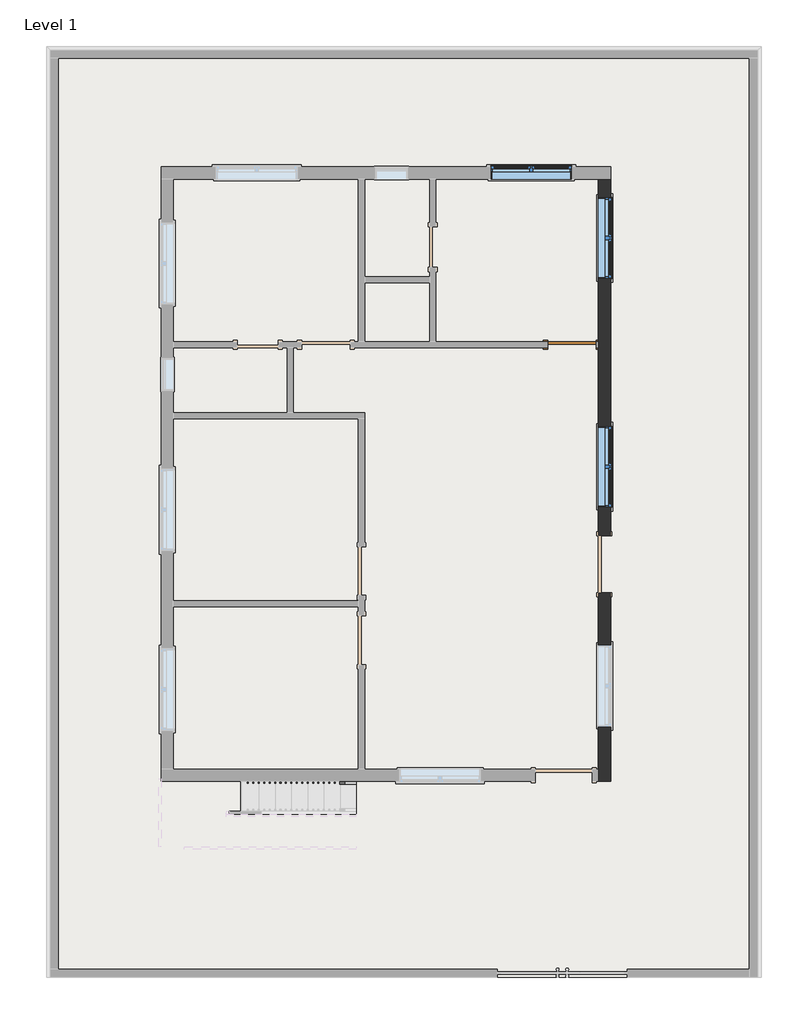
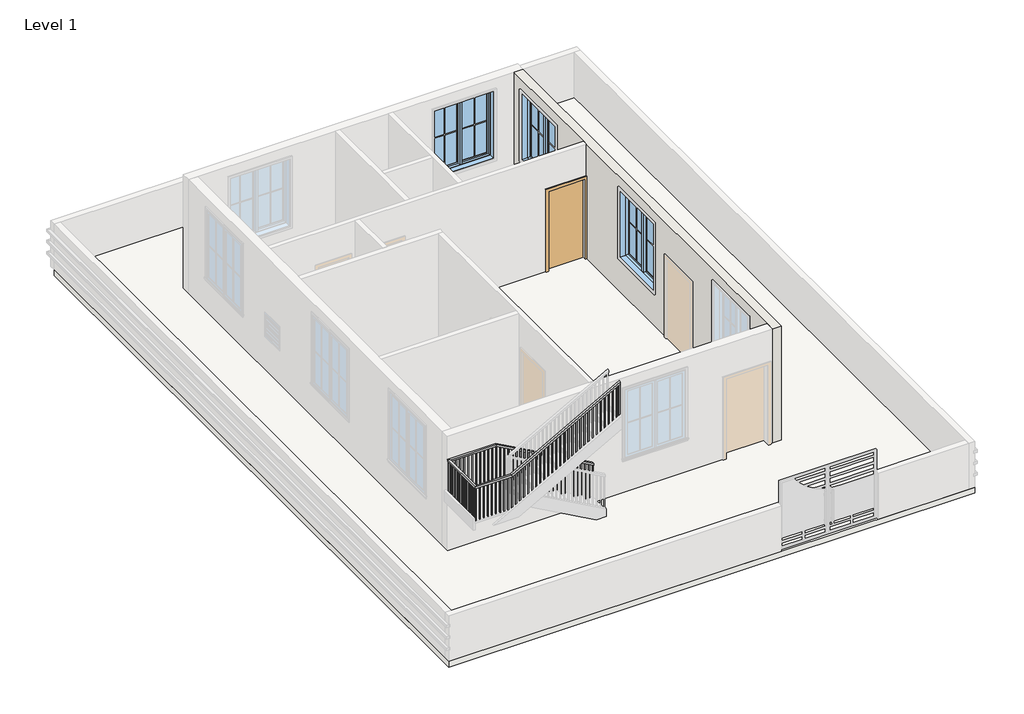
# One storey, part 2 of 3: 3 windows, 1 door, 1 railing, 1 slab, 1 wall.
"""IFC4 building model written with IfcOpenShell, lengths in millimetres."""

from ifc_helpers import new_model, si_unit, frame, origin, place, context, project, spatial, polyline, outline, extrude, faceted_brep, transform, mapped, element, save
from components import single_flush_door_3_e5f9f3c4, window_casement_double_win_5_f93960c7

model = new_model("IFC4")

# Units and contexts
model_context = context("Model", 3, world=origin())
ifc_project = project(units=[si_unit("LENGTHUNIT", "METRE", prefix="MILLI")], contexts=[model_context])

# Site, building, storey
site = spatial("IfcSite", under=ifc_project)
building = spatial("IfcBuilding", under=site)
storey = spatial("IfcBuildingStorey", under=building, Name="Level 1", Elevation=0.0)

# Door
placement = place(None, origin())
single_flush_door_3_shape = single_flush_door_3_e5f9f3c4(model_context)
element("IfcDoor", 1, ObjectType="Single-Flush : DOOR 3'", at=placement, inside=storey, context=model_context, shape_type="MappedRepresentation", body=[
    mapped(single_flush_door_3_shape, transform((2232.6801431, 2878.7566963, 0.0), x_axis=(1.0, 0.0, 0.0), y_axis=(0.0, 1.0, 0.0), z_axis=(0.0, 0.0, 1.0))),
])

# Railing
element("IfcRailing", 2, ObjectType="Handrail - Rectangular", at=placement, inside=storey, context=model_context, shape_type="SolidModel", body=[
    faceted_brep([(-1805.9198569, -5357.1933037, 1083.7333333), (-1805.9198569, -5357.1933037, 1025.620221), (-1805.9198569, -5306.3933037, 1025.620221), (-1805.9198569, -5306.3933037, 1083.7333333), (-4244.3198569, -5357.1933037, 2438.4), (-4257.4834592, -5357.1933037, 2387.6), (-4257.4834592, -5306.3933037, 2387.6), (-4244.3198569, -5306.3933037, 2438.4), (-5412.7198569, -5357.1933037, 2438.4), (-5412.7198569, -5357.1933037, 2387.6), (-5463.5198569, -5306.3933037, 2387.6), (-5463.5198569, -5306.3933037, 2438.4), (-5412.7198569, -6474.7933037, 2438.4), (-5412.7198569, -6474.7933037, 2387.6), (-5463.5198569, -6525.5933037, 2387.6), (-5463.5198569, -6525.5933037, 2438.4), (-4549.1198569, -6474.7933037, 2438.4), (-4535.9562547, -6474.7933037, 2387.6), (-4535.9562547, -6525.5933037, 2387.6), (-4549.1198569, -6525.5933037, 2438.4), (-1805.9198569, -6474.7933037, 3962.4), (-1805.9198569, -6525.5933037, 3962.4), (-1805.9198569, -6525.5933037, 3904.2868876), (-1805.9198569, -6474.7933037, 3904.2868876)], [[[0, 1, 2, 3]], [[1, 0, 4, 5]], [[2, 1, 5, 6]], [[3, 2, 6, 7]], [[0, 3, 7, 4]], [[5, 4, 8, 9]], [[6, 5, 9, 10]], [[7, 6, 10, 11]], [[4, 7, 11, 8]], [[9, 8, 12, 13]], [[10, 9, 13, 14]], [[11, 10, 14, 15]], [[8, 11, 15, 12]], [[13, 12, 16, 17]], [[14, 13, 17, 18]], [[15, 14, 18, 19]], [[12, 15, 19, 16]], [[20, 21, 22, 23]], [[17, 16, 20, 23]], [[18, 17, 23, 22]], [[19, 18, 22, 21]], [[16, 19, 21, 20]]]),
    extrude(outline(polyline([(3867.245221, -1872.5948569), (3856.6618876, -1891.6448569), (2878.6666667, -1891.6448569), (2878.6666667, -1872.5948569), (3867.245221, -1872.5948569)])), frame((0.0, -6509.7183037, 0.0), z_axis=(0.0, 1.0, 0.0), x_axis=(0.0, 0.0, 1.0)), (0.0, 0.0, 1.0), 19.05),
    extrude(outline(polyline([(3810.8007765, -1974.1948569), (3800.2174432, -1993.2448569), (2878.6666667, -1993.2448569), (2878.6666667, -1974.1948569), (3810.8007765, -1974.1948569)])), frame((0.0, -6509.7183037, 0.0), z_axis=(0.0, 1.0, 0.0), x_axis=(0.0, 0.0, 1.0)), (0.0, 0.0, 1.0), 19.05),
    extrude(outline(polyline([(3754.3563321, -2075.7948569), (3743.7729988, -2094.8448569), (2878.6666667, -2094.8448569), (2878.6666667, -2075.7948569), (3754.3563321, -2075.7948569)])), frame((0.0, -6509.7183037, 0.0), z_axis=(0.0, 1.0, 0.0), x_axis=(0.0, 0.0, 1.0)), (0.0, 0.0, 1.0), 19.05),
    extrude(outline(polyline([(3697.9118876, -2177.3948569), (3687.3285543, -2196.4448569), (2709.3333333, -2196.4448569), (2709.3333333, -2177.3948569), (3697.9118876, -2177.3948569)])), frame((0.0, -6509.7183037, 0.0), z_axis=(0.0, 1.0, 0.0), x_axis=(0.0, 0.0, 1.0)), (0.0, 0.0, 1.0), 19.05),
    extrude(outline(polyline([(3641.4674432, -2278.9948569), (3630.8841099, -2298.0448569), (2709.3333333, -2298.0448569), (2709.3333333, -2278.9948569), (3641.4674432, -2278.9948569)])), frame((0.0, -6509.7183037, 0.0), z_axis=(0.0, 1.0, 0.0), x_axis=(0.0, 0.0, 1.0)), (0.0, 0.0, 1.0), 19.05),
    extrude(outline(polyline([(3585.0229988, -2380.5948569), (3574.4396654, -2399.6448569), (2709.3333333, -2399.6448569), (2709.3333333, -2380.5948569), (3585.0229988, -2380.5948569)])), frame((0.0, -6509.7183037, 0.0), z_axis=(0.0, 1.0, 0.0), x_axis=(0.0, 0.0, 1.0)), (0.0, 0.0, 1.0), 19.05),
    extrude(outline(polyline([(3528.5785543, -2482.1948569), (3517.995221, -2501.2448569), (2540.0, -2501.2448569), (2540.0, -2482.1948569), (3528.5785543, -2482.1948569)])), frame((0.0, -6509.7183037, 0.0), z_axis=(0.0, 1.0, 0.0), x_axis=(0.0, 0.0, 1.0)), (0.0, 0.0, 1.0), 19.05),
    extrude(outline(polyline([(3472.1341099, -2583.7948569), (3461.5507765, -2602.8448569), (2540.0, -2602.8448569), (2540.0, -2583.7948569), (3472.1341099, -2583.7948569)])), frame((0.0, -6509.7183037, 0.0), z_axis=(0.0, 1.0, 0.0), x_axis=(0.0, 0.0, 1.0)), (0.0, 0.0, 1.0), 19.05),
    extrude(outline(polyline([(3415.6896654, -2685.3948569), (3405.1063321, -2704.4448569), (2540.0, -2704.4448569), (2540.0, -2685.3948569), (3415.6896654, -2685.3948569)])), frame((0.0, -6509.7183037, 0.0), z_axis=(0.0, 1.0, 0.0), x_axis=(0.0, 0.0, 1.0)), (0.0, 0.0, 1.0), 19.05),
    extrude(outline(polyline([(3359.245221, -2786.9948569), (3348.6618876, -2806.0448569), (2370.6666667, -2806.0448569), (2370.6666667, -2786.9948569), (3359.245221, -2786.9948569)])), frame((0.0, -6509.7183037, 0.0), z_axis=(0.0, 1.0, 0.0), x_axis=(0.0, 0.0, 1.0)), (0.0, 0.0, 1.0), 19.05),
    extrude(outline(polyline([(3302.8007765, -2888.5948569), (3292.2174432, -2907.6448569), (2370.6666667, -2907.6448569), (2370.6666667, -2888.5948569), (3302.8007765, -2888.5948569)])), frame((0.0, -6509.7183037, 0.0), z_axis=(0.0, 1.0, 0.0), x_axis=(0.0, 0.0, 1.0)), (0.0, 0.0, 1.0), 19.05),
    extrude(outline(polyline([(3246.3563321, -2990.1948569), (3235.7729988, -3009.2448569), (2370.6666667, -3009.2448569), (2370.6666667, -2990.1948569), (3246.3563321, -2990.1948569)])), frame((0.0, -6509.7183037, 0.0), z_axis=(0.0, 1.0, 0.0), x_axis=(0.0, 0.0, 1.0)), (0.0, 0.0, 1.0), 19.05),
    extrude(outline(polyline([(3189.9118876, -3091.7948569), (3179.3285543, -3110.8448569), (2201.3333333, -3110.8448569), (2201.3333333, -3091.7948569), (3189.9118876, -3091.7948569)])), frame((0.0, -6509.7183037, 0.0), z_axis=(0.0, 1.0, 0.0), x_axis=(0.0, 0.0, 1.0)), (0.0, 0.0, 1.0), 19.05),
    extrude(outline(polyline([(3133.4674432, -3193.3948569), (3122.8841099, -3212.4448569), (2201.3333333, -3212.4448569), (2201.3333333, -3193.3948569), (3133.4674432, -3193.3948569)])), frame((0.0, -6509.7183037, 0.0), z_axis=(0.0, 1.0, 0.0), x_axis=(0.0, 0.0, 1.0)), (0.0, 0.0, 1.0), 19.05),
    extrude(outline(polyline([(3077.0229988, -3294.9948569), (3066.4396654, -3314.0448569), (2201.3333333, -3314.0448569), (2201.3333333, -3294.9948569), (3077.0229988, -3294.9948569)])), frame((0.0, -6509.7183037, 0.0), z_axis=(0.0, 1.0, 0.0), x_axis=(0.0, 0.0, 1.0)), (0.0, 0.0, 1.0), 19.05),
    extrude(outline(polyline([(3020.5785543, -3396.5948569), (3009.995221, -3415.6448569), (2032.0, -3415.6448569), (2032.0, -3396.5948569), (3020.5785543, -3396.5948569)])), frame((0.0, -6509.7183037, 0.0), z_axis=(0.0, 1.0, 0.0), x_axis=(0.0, 0.0, 1.0)), (0.0, 0.0, 1.0), 19.05),
    extrude(outline(polyline([(2964.1341099, -3498.1948569), (2953.5507765, -3517.2448569), (2032.0, -3517.2448569), (2032.0, -3498.1948569), (2964.1341099, -3498.1948569)])), frame((0.0, -6509.7183037, 0.0), z_axis=(0.0, 1.0, 0.0), x_axis=(0.0, 0.0, 1.0)), (0.0, 0.0, 1.0), 19.05),
    extrude(outline(polyline([(2907.6896654, -3599.7948569), (2897.1063321, -3618.8448569), (2032.0, -3618.8448569), (2032.0, -3599.7948569), (2907.6896654, -3599.7948569)])), frame((0.0, -6509.7183037, 0.0), z_axis=(0.0, 1.0, 0.0), x_axis=(0.0, 0.0, 1.0)), (0.0, 0.0, 1.0), 19.05),
    extrude(outline(polyline([(2851.245221, -3701.3948569), (2840.6618876, -3720.4448569), (1862.6666667, -3720.4448569), (1862.6666667, -3701.3948569), (2851.245221, -3701.3948569)])), frame((0.0, -6509.7183037, 0.0), z_axis=(0.0, 1.0, 0.0), x_axis=(0.0, 0.0, 1.0)), (0.0, 0.0, 1.0), 19.05),
    extrude(outline(polyline([(2794.8007765, -3802.9948569), (2784.2174432, -3822.0448569), (1862.6666667, -3822.0448569), (1862.6666667, -3802.9948569), (2794.8007765, -3802.9948569)])), frame((0.0, -6509.7183037, 0.0), z_axis=(0.0, 1.0, 0.0), x_axis=(0.0, 0.0, 1.0)), (0.0, 0.0, 1.0), 19.05),
    extrude(outline(polyline([(2738.3563321, -3904.5948569), (2727.7729988, -3923.6448569), (1862.6666667, -3923.6448569), (1862.6666667, -3904.5948569), (2738.3563321, -3904.5948569)])), frame((0.0, -6509.7183037, 0.0), z_axis=(0.0, 1.0, 0.0), x_axis=(0.0, 0.0, 1.0)), (0.0, 0.0, 1.0), 19.05),
    extrude(outline(polyline([(2681.9118876, -4006.1948569), (2671.3285543, -4025.2448569), (1693.3333333, -4025.2448569), (1693.3333333, -4006.1948569), (2681.9118876, -4006.1948569)])), frame((0.0, -6509.7183037, 0.0), z_axis=(0.0, 1.0, 0.0), x_axis=(0.0, 0.0, 1.0)), (0.0, 0.0, 1.0), 19.05),
    extrude(outline(polyline([(2625.4674432, -4107.7948569), (2614.8841099, -4126.8448569), (1693.3333333, -4126.8448569), (1693.3333333, -4107.7948569), (2625.4674432, -4107.7948569)])), frame((0.0, -6509.7183037, 0.0), z_axis=(0.0, 1.0, 0.0), x_axis=(0.0, 0.0, 1.0)), (0.0, 0.0, 1.0), 19.05),
    extrude(outline(polyline([(2569.0229988, -4209.3948569), (2558.4396654, -4228.4448569), (1693.3333333, -4228.4448569), (1693.3333333, -4209.3948569), (2569.0229988, -4209.3948569)])), frame((0.0, -6509.7183037, 0.0), z_axis=(0.0, 1.0, 0.0), x_axis=(0.0, 0.0, 1.0)), (0.0, 0.0, 1.0), 19.05),
    extrude(outline(polyline([(2512.5785543, -4310.9948569), (2501.995221, -4330.0448569), (1524.0, -4330.0448569), (1524.0, -4310.9948569), (2512.5785543, -4310.9948569)])), frame((0.0, -6509.7183037, 0.0), z_axis=(0.0, 1.0, 0.0), x_axis=(0.0, 0.0, 1.0)), (0.0, 0.0, 1.0), 19.05),
    extrude(outline(polyline([(2456.1341099, -4412.5948569), (2445.5507765, -4431.6448569), (1524.0, -4431.6448569), (1524.0, -4412.5948569), (2456.1341099, -4412.5948569)])), frame((0.0, -6509.7183037, 0.0), z_axis=(0.0, 1.0, 0.0), x_axis=(0.0, 0.0, 1.0)), (0.0, 0.0, 1.0), 19.05),
    extrude(outline(polyline([(2399.6896654, -4514.1948569), (2389.1063321, -4533.2448569), (1524.0, -4533.2448569), (1524.0, -4514.1948569), (2399.6896654, -4514.1948569)])), frame((0.0, -6509.7183037, 0.0), z_axis=(0.0, 1.0, 0.0), x_axis=(0.0, 0.0, 1.0)), (0.0, 0.0, 1.0), 19.05),
    extrude(outline(polyline([(-4634.8448569, -6509.7183037), (-4634.8448569, -6490.6683037), (-4615.7948569, -6490.6683037), (-4615.7948569, -6509.7183037), (-4634.8448569, -6509.7183037)])), frame((0.0, 0.0, 1524.0), z_axis=(0.0, 0.0, 1.0), x_axis=(1.0, 0.0, 0.0)), (0.0, 0.0, 1.0), 863.6),
    extrude(outline(polyline([(-4736.4448569, -6509.7183037), (-4736.4448569, -6490.6683037), (-4717.3948569, -6490.6683037), (-4717.3948569, -6509.7183037), (-4736.4448569, -6509.7183037)])), frame((0.0, 0.0, 1524.0), z_axis=(0.0, 0.0, 1.0), x_axis=(1.0, 0.0, 0.0)), (0.0, 0.0, 1.0), 863.6),
    extrude(outline(polyline([(-4838.0448569, -6509.7183037), (-4838.0448569, -6490.6683037), (-4818.9948569, -6490.6683037), (-4818.9948569, -6509.7183037), (-4838.0448569, -6509.7183037)])), frame((0.0, 0.0, 1524.0), z_axis=(0.0, 0.0, 1.0), x_axis=(1.0, 0.0, 0.0)), (0.0, 0.0, 1.0), 863.6),
    extrude(outline(polyline([(-4939.6448569, -6509.7183037), (-4939.6448569, -6490.6683037), (-4920.5948569, -6490.6683037), (-4920.5948569, -6509.7183037), (-4939.6448569, -6509.7183037)])), frame((0.0, 0.0, 1524.0), z_axis=(0.0, 0.0, 1.0), x_axis=(1.0, 0.0, 0.0)), (0.0, 0.0, 1.0), 863.6),
    extrude(outline(polyline([(-5041.2448569, -6509.7183037), (-5041.2448569, -6490.6683037), (-5022.1948569, -6490.6683037), (-5022.1948569, -6509.7183037), (-5041.2448569, -6509.7183037)])), frame((0.0, 0.0, 1524.0), z_axis=(0.0, 0.0, 1.0), x_axis=(1.0, 0.0, 0.0)), (0.0, 0.0, 1.0), 863.6),
    extrude(outline(polyline([(-5142.8448569, -6509.7183037), (-5142.8448569, -6490.6683037), (-5123.7948569, -6490.6683037), (-5123.7948569, -6509.7183037), (-5142.8448569, -6509.7183037)])), frame((0.0, 0.0, 1524.0), z_axis=(0.0, 0.0, 1.0), x_axis=(1.0, 0.0, 0.0)), (0.0, 0.0, 1.0), 863.6),
    extrude(outline(polyline([(-5244.4448569, -6509.7183037), (-5244.4448569, -6490.6683037), (-5225.3948569, -6490.6683037), (-5225.3948569, -6509.7183037), (-5244.4448569, -6509.7183037)])), frame((0.0, 0.0, 1524.0), z_axis=(0.0, 0.0, 1.0), x_axis=(1.0, 0.0, 0.0)), (0.0, 0.0, 1.0), 863.6),
    extrude(outline(polyline([(-5346.0448569, -6509.7183037), (-5346.0448569, -6490.6683037), (-5326.9948569, -6490.6683037), (-5326.9948569, -6509.7183037), (-5346.0448569, -6509.7183037)])), frame((0.0, 0.0, 1524.0), z_axis=(0.0, 0.0, 1.0), x_axis=(1.0, 0.0, 0.0)), (0.0, 0.0, 1.0), 863.6),
    extrude(outline(polyline([(-5447.6448569, -6439.8683037), (-5428.5948569, -6439.8683037), (-5428.5948569, -6458.9183037), (-5447.6448569, -6458.9183037), (-5447.6448569, -6439.8683037)])), frame((0.0, 0.0, 1524.0), z_axis=(0.0, 0.0, 1.0), x_axis=(1.0, 0.0, 0.0)), (0.0, 0.0, 1.0), 863.6),
    extrude(outline(polyline([(-5447.6448569, -6338.2683037), (-5428.5948569, -6338.2683037), (-5428.5948569, -6357.3183037), (-5447.6448569, -6357.3183037), (-5447.6448569, -6338.2683037)])), frame((0.0, 0.0, 1524.0), z_axis=(0.0, 0.0, 1.0), x_axis=(1.0, 0.0, 0.0)), (0.0, 0.0, 1.0), 863.6),
    extrude(outline(polyline([(-5447.6448569, -6236.6683037), (-5428.5948569, -6236.6683037), (-5428.5948569, -6255.7183037), (-5447.6448569, -6255.7183037), (-5447.6448569, -6236.6683037)])), frame((0.0, 0.0, 1524.0), z_axis=(0.0, 0.0, 1.0), x_axis=(1.0, 0.0, 0.0)), (0.0, 0.0, 1.0), 863.6),
    extrude(outline(polyline([(-5447.6448569, -6135.0683037), (-5428.5948569, -6135.0683037), (-5428.5948569, -6154.1183037), (-5447.6448569, -6154.1183037), (-5447.6448569, -6135.0683037)])), frame((0.0, 0.0, 1524.0), z_axis=(0.0, 0.0, 1.0), x_axis=(1.0, 0.0, 0.0)), (0.0, 0.0, 1.0), 863.6),
    extrude(outline(polyline([(-5447.6448569, -6033.4683037), (-5428.5948569, -6033.4683037), (-5428.5948569, -6052.5183037), (-5447.6448569, -6052.5183037), (-5447.6448569, -6033.4683037)])), frame((0.0, 0.0, 1524.0), z_axis=(0.0, 0.0, 1.0), x_axis=(1.0, 0.0, 0.0)), (0.0, 0.0, 1.0), 863.6),
    extrude(outline(polyline([(-5447.6448569, -5931.8683037), (-5428.5948569, -5931.8683037), (-5428.5948569, -5950.9183037), (-5447.6448569, -5950.9183037), (-5447.6448569, -5931.8683037)])), frame((0.0, 0.0, 1524.0), z_axis=(0.0, 0.0, 1.0), x_axis=(1.0, 0.0, 0.0)), (0.0, 0.0, 1.0), 863.6),
    extrude(outline(polyline([(-5447.6448569, -5830.2683037), (-5428.5948569, -5830.2683037), (-5428.5948569, -5849.3183037), (-5447.6448569, -5849.3183037), (-5447.6448569, -5830.2683037)])), frame((0.0, 0.0, 1524.0), z_axis=(0.0, 0.0, 1.0), x_axis=(1.0, 0.0, 0.0)), (0.0, 0.0, 1.0), 863.6),
    extrude(outline(polyline([(-5447.6448569, -5728.6683037), (-5428.5948569, -5728.6683037), (-5428.5948569, -5747.7183037), (-5447.6448569, -5747.7183037), (-5447.6448569, -5728.6683037)])), frame((0.0, 0.0, 1524.0), z_axis=(0.0, 0.0, 1.0), x_axis=(1.0, 0.0, 0.0)), (0.0, 0.0, 1.0), 863.6),
    extrude(outline(polyline([(-5447.6448569, -5627.0683037), (-5428.5948569, -5627.0683037), (-5428.5948569, -5646.1183037), (-5447.6448569, -5646.1183037), (-5447.6448569, -5627.0683037)])), frame((0.0, 0.0, 1524.0), z_axis=(0.0, 0.0, 1.0), x_axis=(1.0, 0.0, 0.0)), (0.0, 0.0, 1.0), 863.6),
    extrude(outline(polyline([(-5447.6448569, -5525.4683037), (-5428.5948569, -5525.4683037), (-5428.5948569, -5544.5183037), (-5447.6448569, -5544.5183037), (-5447.6448569, -5525.4683037)])), frame((0.0, 0.0, 1524.0), z_axis=(0.0, 0.0, 1.0), x_axis=(1.0, 0.0, 0.0)), (0.0, 0.0, 1.0), 863.6),
    extrude(outline(polyline([(-5447.6448569, -5423.8683037), (-5428.5948569, -5423.8683037), (-5428.5948569, -5442.9183037), (-5447.6448569, -5442.9183037), (-5447.6448569, -5423.8683037)])), frame((0.0, 0.0, 1524.0), z_axis=(0.0, 0.0, 1.0), x_axis=(1.0, 0.0, 0.0)), (0.0, 0.0, 1.0), 863.6),
    extrude(outline(polyline([(-5352.3948569, -5322.2683037), (-5352.3948569, -5341.3183037), (-5371.4448569, -5341.3183037), (-5371.4448569, -5322.2683037), (-5352.3948569, -5322.2683037)])), frame((0.0, 0.0, 1524.0), z_axis=(0.0, 0.0, 1.0), x_axis=(1.0, 0.0, 0.0)), (0.0, 0.0, 1.0), 863.6),
    extrude(outline(polyline([(-5250.7948569, -5322.2683037), (-5250.7948569, -5341.3183037), (-5269.8448569, -5341.3183037), (-5269.8448569, -5322.2683037), (-5250.7948569, -5322.2683037)])), frame((0.0, 0.0, 1524.0), z_axis=(0.0, 0.0, 1.0), x_axis=(1.0, 0.0, 0.0)), (0.0, 0.0, 1.0), 863.6),
    extrude(outline(polyline([(-5149.1948569, -5322.2683037), (-5149.1948569, -5341.3183037), (-5168.2448569, -5341.3183037), (-5168.2448569, -5322.2683037), (-5149.1948569, -5322.2683037)])), frame((0.0, 0.0, 1524.0), z_axis=(0.0, 0.0, 1.0), x_axis=(1.0, 0.0, 0.0)), (0.0, 0.0, 1.0), 863.6),
    extrude(outline(polyline([(-5047.5948569, -5322.2683037), (-5047.5948569, -5341.3183037), (-5066.6448569, -5341.3183037), (-5066.6448569, -5322.2683037), (-5047.5948569, -5322.2683037)])), frame((0.0, 0.0, 1524.0), z_axis=(0.0, 0.0, 1.0), x_axis=(1.0, 0.0, 0.0)), (0.0, 0.0, 1.0), 863.6),
    extrude(outline(polyline([(-4945.9948569, -5322.2683037), (-4945.9948569, -5341.3183037), (-4965.0448569, -5341.3183037), (-4965.0448569, -5322.2683037), (-4945.9948569, -5322.2683037)])), frame((0.0, 0.0, 1524.0), z_axis=(0.0, 0.0, 1.0), x_axis=(1.0, 0.0, 0.0)), (0.0, 0.0, 1.0), 863.6),
    extrude(outline(polyline([(-4844.3948569, -5322.2683037), (-4844.3948569, -5341.3183037), (-4863.4448569, -5341.3183037), (-4863.4448569, -5322.2683037), (-4844.3948569, -5322.2683037)])), frame((0.0, 0.0, 1524.0), z_axis=(0.0, 0.0, 1.0), x_axis=(1.0, 0.0, 0.0)), (0.0, 0.0, 1.0), 863.6),
    extrude(outline(polyline([(-4742.7948569, -5322.2683037), (-4742.7948569, -5341.3183037), (-4761.8448569, -5341.3183037), (-4761.8448569, -5322.2683037), (-4742.7948569, -5322.2683037)])), frame((0.0, 0.0, 1524.0), z_axis=(0.0, 0.0, 1.0), x_axis=(1.0, 0.0, 0.0)), (0.0, 0.0, 1.0), 863.6),
    extrude(outline(polyline([(-4641.1948569, -5322.2683037), (-4641.1948569, -5341.3183037), (-4660.2448569, -5341.3183037), (-4660.2448569, -5322.2683037), (-4641.1948569, -5322.2683037)])), frame((0.0, 0.0, 1524.0), z_axis=(0.0, 0.0, 1.0), x_axis=(1.0, 0.0, 0.0)), (0.0, 0.0, 1.0), 863.6),
    extrude(outline(polyline([(-4539.5948569, -5322.2683037), (-4539.5948569, -5341.3183037), (-4558.6448569, -5341.3183037), (-4558.6448569, -5322.2683037), (-4539.5948569, -5322.2683037)])), frame((0.0, 0.0, 1524.0), z_axis=(0.0, 0.0, 1.0), x_axis=(1.0, 0.0, 0.0)), (0.0, 0.0, 1.0), 863.6),
    extrude(outline(polyline([(-4437.9948569, -5322.2683037), (-4437.9948569, -5341.3183037), (-4457.0448569, -5341.3183037), (-4457.0448569, -5322.2683037), (-4437.9948569, -5322.2683037)])), frame((0.0, 0.0, 1524.0), z_axis=(0.0, 0.0, 1.0), x_axis=(1.0, 0.0, 0.0)), (0.0, 0.0, 1.0), 863.6),
    extrude(outline(polyline([(-4336.3948569, -5322.2683037), (-4336.3948569, -5341.3183037), (-4355.4448569, -5341.3183037), (-4355.4448569, -5322.2683037), (-4336.3948569, -5322.2683037)])), frame((0.0, 0.0, 1524.0), z_axis=(0.0, 0.0, 1.0), x_axis=(1.0, 0.0, 0.0)), (0.0, 0.0, 1.0), 863.6),
    extrude(outline(polyline([(2374.995221, -4234.7948569), (2385.5785543, -4253.8448569), (1524.0, -4253.8448569), (1524.0, -4234.7948569), (2374.995221, -4234.7948569)])), frame((0.0, -5341.3183037, 0.0), z_axis=(0.0, 1.0, 0.0), x_axis=(0.0, 0.0, 1.0)), (0.0, 0.0, 1.0), 19.05),
    extrude(outline(polyline([(2318.5507765, -4133.1948569), (2329.1341099, -4152.2448569), (1354.6666667, -4152.2448569), (1354.6666667, -4133.1948569), (2318.5507765, -4133.1948569)])), frame((0.0, -5341.3183037, 0.0), z_axis=(0.0, 1.0, 0.0), x_axis=(0.0, 0.0, 1.0)), (0.0, 0.0, 1.0), 19.05),
    extrude(outline(polyline([(2262.1063321, -4031.5948569), (2272.6896654, -4050.6448569), (1354.6666667, -4050.6448569), (1354.6666667, -4031.5948569), (2262.1063321, -4031.5948569)])), frame((0.0, -5341.3183037, 0.0), z_axis=(0.0, 1.0, 0.0), x_axis=(0.0, 0.0, 1.0)), (0.0, 0.0, 1.0), 19.05),
    extrude(outline(polyline([(2205.6618876, -3929.9948569), (2216.245221, -3949.0448569), (1354.6666667, -3949.0448569), (1354.6666667, -3929.9948569), (2205.6618876, -3929.9948569)])), frame((0.0, -5341.3183037, 0.0), z_axis=(0.0, 1.0, 0.0), x_axis=(0.0, 0.0, 1.0)), (0.0, 0.0, 1.0), 19.05),
    extrude(outline(polyline([(2149.2174432, -3828.3948569), (2159.8007765, -3847.4448569), (1185.3333333, -3847.4448569), (1185.3333333, -3828.3948569), (2149.2174432, -3828.3948569)])), frame((0.0, -5341.3183037, 0.0), z_axis=(0.0, 1.0, 0.0), x_axis=(0.0, 0.0, 1.0)), (0.0, 0.0, 1.0), 19.05),
    extrude(outline(polyline([(2092.7729988, -3726.7948569), (2103.3563321, -3745.8448569), (1185.3333333, -3745.8448569), (1185.3333333, -3726.7948569), (2092.7729988, -3726.7948569)])), frame((0.0, -5341.3183037, 0.0), z_axis=(0.0, 1.0, 0.0), x_axis=(0.0, 0.0, 1.0)), (0.0, 0.0, 1.0), 19.05),
    extrude(outline(polyline([(2036.3285543, -3625.1948569), (2046.9118876, -3644.2448569), (1185.3333333, -3644.2448569), (1185.3333333, -3625.1948569), (2036.3285543, -3625.1948569)])), frame((0.0, -5341.3183037, 0.0), z_axis=(0.0, 1.0, 0.0), x_axis=(0.0, 0.0, 1.0)), (0.0, 0.0, 1.0), 19.05),
    extrude(outline(polyline([(1979.8841099, -3523.5948569), (1990.4674432, -3542.6448569), (1016.0, -3542.6448569), (1016.0, -3523.5948569), (1979.8841099, -3523.5948569)])), frame((0.0, -5341.3183037, 0.0), z_axis=(0.0, 1.0, 0.0), x_axis=(0.0, 0.0, 1.0)), (0.0, 0.0, 1.0), 19.05),
    extrude(outline(polyline([(1923.4396654, -3421.9948569), (1934.0229988, -3441.0448569), (1016.0, -3441.0448569), (1016.0, -3421.9948569), (1923.4396654, -3421.9948569)])), frame((0.0, -5341.3183037, 0.0), z_axis=(0.0, 1.0, 0.0), x_axis=(0.0, 0.0, 1.0)), (0.0, 0.0, 1.0), 19.05),
    extrude(outline(polyline([(1866.995221, -3320.3948569), (1877.5785543, -3339.4448569), (1016.0, -3339.4448569), (1016.0, -3320.3948569), (1866.995221, -3320.3948569)])), frame((0.0, -5341.3183037, 0.0), z_axis=(0.0, 1.0, 0.0), x_axis=(0.0, 0.0, 1.0)), (0.0, 0.0, 1.0), 19.05),
    extrude(outline(polyline([(1810.5507765, -3218.7948569), (1821.1341099, -3237.8448569), (846.6666667, -3237.8448569), (846.6666667, -3218.7948569), (1810.5507765, -3218.7948569)])), frame((0.0, -5341.3183037, 0.0), z_axis=(0.0, 1.0, 0.0), x_axis=(0.0, 0.0, 1.0)), (0.0, 0.0, 1.0), 19.05),
    extrude(outline(polyline([(1754.1063321, -3117.1948569), (1764.6896654, -3136.2448569), (846.6666667, -3136.2448569), (846.6666667, -3117.1948569), (1754.1063321, -3117.1948569)])), frame((0.0, -5341.3183037, 0.0), z_axis=(0.0, 1.0, 0.0), x_axis=(0.0, 0.0, 1.0)), (0.0, 0.0, 1.0), 19.05),
    extrude(outline(polyline([(1697.6618876, -3015.5948569), (1708.245221, -3034.6448569), (846.6666667, -3034.6448569), (846.6666667, -3015.5948569), (1697.6618876, -3015.5948569)])), frame((0.0, -5341.3183037, 0.0), z_axis=(0.0, 1.0, 0.0), x_axis=(0.0, 0.0, 1.0)), (0.0, 0.0, 1.0), 19.05),
    extrude(outline(polyline([(1641.2174432, -2913.9948569), (1651.8007765, -2933.0448569), (677.3333333, -2933.0448569), (677.3333333, -2913.9948569), (1641.2174432, -2913.9948569)])), frame((0.0, -5341.3183037, 0.0), z_axis=(0.0, 1.0, 0.0), x_axis=(0.0, 0.0, 1.0)), (0.0, 0.0, 1.0), 19.05),
    extrude(outline(polyline([(1584.7729988, -2812.3948569), (1595.3563321, -2831.4448569), (677.3333333, -2831.4448569), (677.3333333, -2812.3948569), (1584.7729988, -2812.3948569)])), frame((0.0, -5341.3183037, 0.0), z_axis=(0.0, 1.0, 0.0), x_axis=(0.0, 0.0, 1.0)), (0.0, 0.0, 1.0), 19.05),
    extrude(outline(polyline([(1528.3285543, -2710.7948569), (1538.9118876, -2729.8448569), (677.3333333, -2729.8448569), (677.3333333, -2710.7948569), (1528.3285543, -2710.7948569)])), frame((0.0, -5341.3183037, 0.0), z_axis=(0.0, 1.0, 0.0), x_axis=(0.0, 0.0, 1.0)), (0.0, 0.0, 1.0), 19.05),
    extrude(outline(polyline([(1471.8841099, -2609.1948569), (1482.4674432, -2628.2448569), (508.0, -2628.2448569), (508.0, -2609.1948569), (1471.8841099, -2609.1948569)])), frame((0.0, -5341.3183037, 0.0), z_axis=(0.0, 1.0, 0.0), x_axis=(0.0, 0.0, 1.0)), (0.0, 0.0, 1.0), 19.05),
    extrude(outline(polyline([(1415.4396654, -2507.5948569), (1426.0229988, -2526.6448569), (508.0, -2526.6448569), (508.0, -2507.5948569), (1415.4396654, -2507.5948569)])), frame((0.0, -5341.3183037, 0.0), z_axis=(0.0, 1.0, 0.0), x_axis=(0.0, 0.0, 1.0)), (0.0, 0.0, 1.0), 19.05),
    extrude(outline(polyline([(1358.995221, -2405.9948569), (1369.5785543, -2425.0448569), (508.0, -2425.0448569), (508.0, -2405.9948569), (1358.995221, -2405.9948569)])), frame((0.0, -5341.3183037, 0.0), z_axis=(0.0, 1.0, 0.0), x_axis=(0.0, 0.0, 1.0)), (0.0, 0.0, 1.0), 19.05),
    extrude(outline(polyline([(1302.5507765, -2304.3948569), (1313.1341099, -2323.4448569), (338.6666667, -2323.4448569), (338.6666667, -2304.3948569), (1302.5507765, -2304.3948569)])), frame((0.0, -5341.3183037, 0.0), z_axis=(0.0, 1.0, 0.0), x_axis=(0.0, 0.0, 1.0)), (0.0, 0.0, 1.0), 19.05),
    extrude(outline(polyline([(1246.1063321, -2202.7948569), (1256.6896654, -2221.8448569), (338.6666667, -2221.8448569), (338.6666667, -2202.7948569), (1246.1063321, -2202.7948569)])), frame((0.0, -5341.3183037, 0.0), z_axis=(0.0, 1.0, 0.0), x_axis=(0.0, 0.0, 1.0)), (0.0, 0.0, 1.0), 19.05),
    extrude(outline(polyline([(1189.6618876, -2101.1948569), (1200.245221, -2120.2448569), (338.6666667, -2120.2448569), (338.6666667, -2101.1948569), (1189.6618876, -2101.1948569)])), frame((0.0, -5341.3183037, 0.0), z_axis=(0.0, 1.0, 0.0), x_axis=(0.0, 0.0, 1.0)), (0.0, 0.0, 1.0), 19.05),
    extrude(outline(polyline([(1133.2174432, -1999.5948569), (1143.8007765, -2018.6448569), (169.3333333, -2018.6448569), (169.3333333, -1999.5948569), (1133.2174432, -1999.5948569)])), frame((0.0, -5341.3183037, 0.0), z_axis=(0.0, 1.0, 0.0), x_axis=(0.0, 0.0, 1.0)), (0.0, 0.0, 1.0), 19.05),
    extrude(outline(polyline([(1076.7729988, -1897.9948569), (1087.3563321, -1917.0448569), (169.3333333, -1917.0448569), (169.3333333, -1897.9948569), (1076.7729988, -1897.9948569)])), frame((0.0, -5341.3183037, 0.0), z_axis=(0.0, 1.0, 0.0), x_axis=(0.0, 0.0, 1.0)), (0.0, 0.0, 1.0), 19.05),
    extrude(outline(polyline([(-5447.6448569, -6490.6683037), (-5428.5948569, -6490.6683037), (-5428.5948569, -6509.7183037), (-5447.6448569, -6509.7183037), (-5447.6448569, -6490.6683037)])), frame((0.0, 0.0, 1524.0), z_axis=(0.0, 0.0, 1.0), x_axis=(1.0, 0.0, 0.0)), (0.0, 0.0, 1.0), 863.6),
    extrude(outline(polyline([(-5428.5948569, -5322.2683037), (-5428.5948569, -5341.3183037), (-5447.6448569, -5341.3183037), (-5447.6448569, -5322.2683037), (-5428.5948569, -5322.2683037)])), frame((0.0, 0.0, 1524.0), z_axis=(0.0, 0.0, 1.0), x_axis=(1.0, 0.0, 0.0)), (0.0, 0.0, 1.0), 863.6),
    extrude(outline(polyline([(3904.2868876, -1805.9198569), (3893.7035543, -1824.9698569), (2878.6666667, -1824.9698569), (2878.6666667, -1805.9198569), (3904.2868876, -1805.9198569)])), frame((0.0, -6509.7183037, 0.0), z_axis=(0.0, 1.0, 0.0), x_axis=(0.0, 0.0, 1.0)), (0.0, 0.0, 1.0), 19.05),
    extrude(outline(polyline([(1025.620221, -1805.9198569), (1036.2035543, -1824.9698569), (169.3333333, -1824.9698569), (169.3333333, -1805.9198569), (1025.620221, -1805.9198569)])), frame((0.0, -5341.3183037, 0.0), z_axis=(0.0, 1.0, 0.0), x_axis=(0.0, 0.0, 1.0)), (0.0, 0.0, 1.0), 19.05),
])

# Slab
element("IfcSlab", 3, ObjectType="FLOOR 6\"", at=placement, inside=storey, context=model_context, shape_type="SweptSolid", body=[
    extrude(outline(polyline([(5712.5561924, 8248.1249463), (5712.5561924, -8973.0750537), (-7546.2438076, -8973.0750537), (-7546.2438076, 8248.1249463), (5712.5561924, 8248.1249463)])), frame((0.0, 0.0, -152.4), z_axis=(0.0, 0.0, 1.0), x_axis=(1.0, 0.0, 0.0)), (0.0, 0.0, 1.0), 152.4),
])

# Wall
element("IfcWall", 4, ObjectType="WALL 9\"", at=placement, inside=storey, context=model_context, shape_type="Brep", body=[
    faceted_brep([(2727.9801431, -1769.4433037, 2133.6), (2727.9801431, -1769.4433037, 0.0), (2727.9801431, -5077.7933037, 0.0), (2727.9801431, -5306.3933037, 0.0), (2727.9801431, -5306.3933037, 3048.0), (2727.9801431, -5077.7933037, 3048.0), (2727.9801431, 2821.6066963, 3048.0), (2727.9801431, 2935.9066963, 3048.0), (2727.9801431, 5983.9066963, 3048.0), (2727.9801431, 5983.9066963, 0.0), (2727.9801431, 2935.9066963, 0.0), (2727.9801431, 2821.6066963, 0.0), (2727.9801431, -702.6433037, 0.0), (2727.9801431, -702.6433037, 2133.6), (2727.9801431, 4117.0066963, 2743.2), (2727.9801431, 4117.0066963, 914.4), (2727.9801431, 5641.0066963, 914.4), (2727.9801431, 5641.0066963, 2743.2), (2727.9801431, -169.2433037, 2743.2), (2727.9801431, -169.2433037, 914.4), (2727.9801431, 1354.7566963, 914.4), (2727.9801431, 1354.7566963, 2743.2), (2727.9801431, -4277.6933037, 2743.2), (2727.9801431, -4277.6933037, 914.4), (2727.9801431, -2753.6933037, 914.4), (2727.9801431, -2753.6933037, 2743.2), (2956.5801431, -5306.3933037, 0.0), (2956.5801431, -1769.4433037, 0.0), (2956.5801431, -1769.4433037, 2133.6), (2956.5801431, -702.6433037, 2133.6), (2956.5801431, -702.6433037, 0.0), (2956.5801431, 5983.9066963, 0.0), (2956.5801431, 5983.9066963, 3048.0), (2956.5801431, -5306.3933037, 3048.0), (2956.5801431, 4117.0066963, 2743.2), (2956.5801431, 5641.0066963, 2743.2), (2956.5801431, 5641.0066963, 914.4), (2956.5801431, 4117.0066963, 914.4), (2956.5801431, -169.2433037, 2743.2), (2956.5801431, 1354.7566963, 2743.2), (2956.5801431, 1354.7566963, 914.4), (2956.5801431, -169.2433037, 914.4), (2956.5801431, -4277.6933037, 2743.2), (2956.5801431, -2753.6933037, 2743.2), (2956.5801431, -2753.6933037, 914.4), (2956.5801431, -4277.6933037, 914.4)], [[[0, 1, 2, 3, 4, 5, 6, 7, 8, 9, 10, 11, 12, 13], [14, 15, 16, 17], [18, 19, 20, 21], [22, 23, 24, 25]], [[26, 27, 28, 29, 30, 31, 32, 33], [34, 35, 36, 37], [38, 39, 40, 41], [42, 43, 44, 45]], [[3, 2, 1, 27, 26]], [[12, 11, 10, 9, 31, 30]], [[9, 8, 32, 31]], [[4, 3, 26, 33]], [[15, 14, 34, 37]], [[16, 15, 37, 36]], [[17, 16, 36, 35]], [[14, 17, 35, 34]], [[19, 18, 38, 41]], [[20, 19, 41, 40]], [[21, 20, 40, 39]], [[18, 21, 39, 38]], [[23, 22, 42, 45]], [[24, 23, 45, 44]], [[25, 24, 44, 43]], [[22, 25, 43, 42]], [[28, 27, 1, 0]], [[29, 28, 0, 13]], [[30, 29, 13, 12]], [[8, 7, 6, 5, 4, 33, 32]]]),
])

# Windows
window_casement_double_win_5_shape = window_casement_double_win_5_f93960c7(model_context)
element("IfcWindow", 5, ObjectType="Window-Casement-Double : WIN 5'", at=placement, inside=storey, context=model_context, shape_type="MappedRepresentation", body=[
    mapped(window_casement_double_win_5_shape, transform((2842.2801431, 4879.0066963, 0.0), x_axis=(0.0, -1.0, 0.0), y_axis=(1.0, 0.0, 0.0), z_axis=(0.0, 0.0, 1.0))),
])
element("IfcWindow", 6, ObjectType="Window-Casement-Double : WIN 5'", at=placement, inside=storey, context=model_context, shape_type="MappedRepresentation", body=[
    mapped(window_casement_double_win_5_shape, transform((2842.2801431, 592.7566963, 0.0), x_axis=(0.0, -1.0, 0.0), y_axis=(1.0, 0.0, 0.0), z_axis=(0.0, 0.0, 1.0))),
])
element("IfcWindow", 7, ObjectType="Window-Casement-Double : WIN 5'", at=placement, inside=storey, context=model_context, shape_type="MappedRepresentation", body=[
    mapped(window_casement_double_win_5_shape, transform((1470.6801431, 6098.2066963, 0.0), x_axis=(1.0, 0.0, 0.0), y_axis=(0.0, 1.0, 0.0), z_axis=(0.0, 0.0, 1.0))),
])

save(model, "model.ifc")

# Revit data of these elements
# Type "Single-Flush : DOOR 3'"
#   Type Mark = "8"
#   Construction Type Id = "MDOOR"
#   Assembly Code = "C1020"
#   Analytic Construction = "Metal"
#   Thickness = 0' - 2"
#   Heat Transfer Coefficient (U) = 0.651978 BTU/(h·ft²·°F)
#   Height = 7' - 0"
#   Trim Projection Ext = 0' - 1"
#   Trim Projection Int = 0' - 1"
#   Trim Width = 0' - 3"
#   Width = 3' - 0"
#   Define Thermal Properties by = 1
#   Door Material = Door - Panel
#   Frame Material = Door - Frame
#   Visual Light Transmittance = 0
#   Solar Heat Gain Coefficient = 0
#   Function = (empty or 0)
#   Wall Closure = (empty or 0)
# Type "Handrail - Rectangular"
#   Assembly Code = "C2010400"
#   built-in parameter 1008612 = 0.0416667 (stored number, unit not read)
#   built-in parameter 1008611 = 0.0416667 (stored number, unit not read)
#   built-in parameter 1008609 = 0.333333 (stored number, unit not read)
#   built-in parameter 1008604 = 0.166667 (stored number, unit not read)
#   built-in parameter 1008603 = 0.166667 (stored number, unit not read)
#   Railing Height = 3' - 0"
#   built-in parameter 1008630 = 2
#   built-in parameter 1008610 = 2
#   built-in parameter 1008618 = Baluster - Square : 3/4"
# Type "FLOOR 6\""
#   Assembly Code = "B1010"
#   Function = 0
#   Layers, outside or top first: 0' - 6" no material (function 1)
# Type "WALL 9\""
#   Assembly Code = "B2010"
#   Layers, outside or top first: 0' - 9" no material (function 1)
# Type "Window-Casement-Double : WIN 5'"
#   Type Mark = "20"
#   Fire Rating = "0.5h"
#   Assembly Code = "B2020100"
#   Analytic Construction = "Double glazing - domestic"
#   Frame Extension [instance default] = 0' - 0 1/4"
#   Window Inset [instance default] = 0' - 0"
#   Wall Thickness [instance default] = 0' - 6"
#   Interior Wall Closure [instance default] = 0' - 2 1/4"
#   Half Width = 2' - 6"
#   Visual Light Transmittance = 0.81
#   Thermal Resistance (R) = 1.8146 (h·ft²·°F)/BTU
#   Solar Heat Gain Coefficient = 0.76
#   Rough Width = 5' - 0 1/2"
#   Rough Height = 6' - 0 1/2"
#   Height = 6' - 0"
#   Heat Transfer Coefficient (U) = 0.5511 BTU/(h·ft²·°F)
#   Exterior Wall Closure [instance default] = 0' - 1 1/4"
#   Extension Jamb [instance default] = 0' - 2 1/4"
#   Default Sill Height = 3' - 0"
#   Width = 5' - 0"
#   Muntin Visibility = yes
#   Interior Trim Visibility [instance default] = yes
#   Exterior Trim Visibility [instance default] = yes
#   Extension Jamb Visibility [instance default] = yes
#   Interior Trim Material = Wood - Stained
#   Muntin Pattern = Muntin Pattern_2x2 : Muntin Pattern_2x2
#   Interior Trim = Trim-Window-Interior-Flat : Picture Frame
#   Interior Frame Material = Wood - Stained
#   Glass Panel Material = Glass
#   Exterior Trim Material = Clad - White
#   Exterior Trim = Trim-Window-Exterior-Flat : with Sill
#   Exterior Frame Material = Clad - White
#   Wall Closure = (empty or 0)
# Element 1 (IfcDoor, "Single-Flush : DOOR 3'")
#   Phase Created = New Construction
#   Materials on its faces: "Door - Frame", "Door - Panel"
# Element 2 (IfcRailing, "Handrail - Rectangular")
#   Phase Created = New Construction
# Element 3 (IfcSlab, "FLOOR 6\"")
#   Height Offset From Level = 0' - 0"
#   Phase Created = New Construction
#   Materials on its faces: "Parking Stripe", "Default Floor", "Wood - Stained"
# Element 4 (IfcWall, "WALL 9\"")
#   Top Offset = 0' - 0"
#   Base Offset = 0' - 0"
#   Unconnected Height = 10' - 0"
#   wall height = 10' - 0"
#   Phase Created = New Construction
#   Base Constraint = Level 1
#   Materials on its faces: "Default Wall", "Cherry"
# Element 5 (IfcWindow, "Window-Casement-Double : WIN 5'")
#   Mark = "4"
#   Window Inset = 0' - 0"
#   Interior Wall Closure = 0' - 2 1/4"
#   Frame Extension = 0' - 0 1/4"
#   Exterior Wall Closure = 0' - 1 1/4"
#   Interior Trim Visibility = yes
#   Exterior Trim Visibility = yes
#   Phase Created = New Construction
#   Materials on its faces: "Wood - Stained", "Glass", "Clad - White"
# Element 6 (IfcWindow, "Window-Casement-Double : WIN 5'")
#   Mark = "5"
#   Window Inset = 0' - 0"
#   Interior Wall Closure = 0' - 2 1/4"
#   Frame Extension = 0' - 0 1/4"
#   Exterior Wall Closure = 0' - 1 1/4"
#   Interior Trim Visibility = yes
#   Exterior Trim Visibility = yes
#   Phase Created = New Construction
#   Materials on its faces: "Wood - Stained", "Glass", "Clad - White"
# Element 7 (IfcWindow, "Window-Casement-Double : WIN 5'")
#   Mark = "8"
#   Window Inset = 0' - 0"
#   Interior Wall Closure = 0' - 2 1/4"
#   Frame Extension = 0' - 0 1/4"
#   Exterior Wall Closure = 0' - 1 1/4"
#   Interior Trim Visibility = yes
#   Exterior Trim Visibility = yes
#   Phase Created = New Construction
#   Materials on its faces: "Wood - Stained", "Glass", "Clad - White"
# Materials
#   "Door - Panel": class "Wood", colour RGB 210 159 95, transparency 0, Cost = 0
#   "Door - Frame": colour RGB 118 70 51, transparency 0, Cost = 0
#   "Wood - Stained": class "Wood", colour RGB 224 178 126, transparency 0, Cost = 0
#   "Glass": class "Glass", colour RGB 0 128 192, transparency 0.75, Description = "Soda Lime Glass", Cost = 0
#   "Clad - White": class "Wood", colour RGB 242 242 238, transparency 0, Cost = 0
#   "Parking Stripe": class "Paint", colour RGB 250 250 91, transparency 0, Cost = 0
#   "Default Floor": colour RGB 128 128 128, transparency 0, Cost = 0
#   "Default Wall": colour RGB 128 128 128, transparency 0, Cost = 0
#   "Cherry": class "Wood", colour RGB 226 177 128, transparency 0, Description = "Prunus Serotina", Cost = 0
